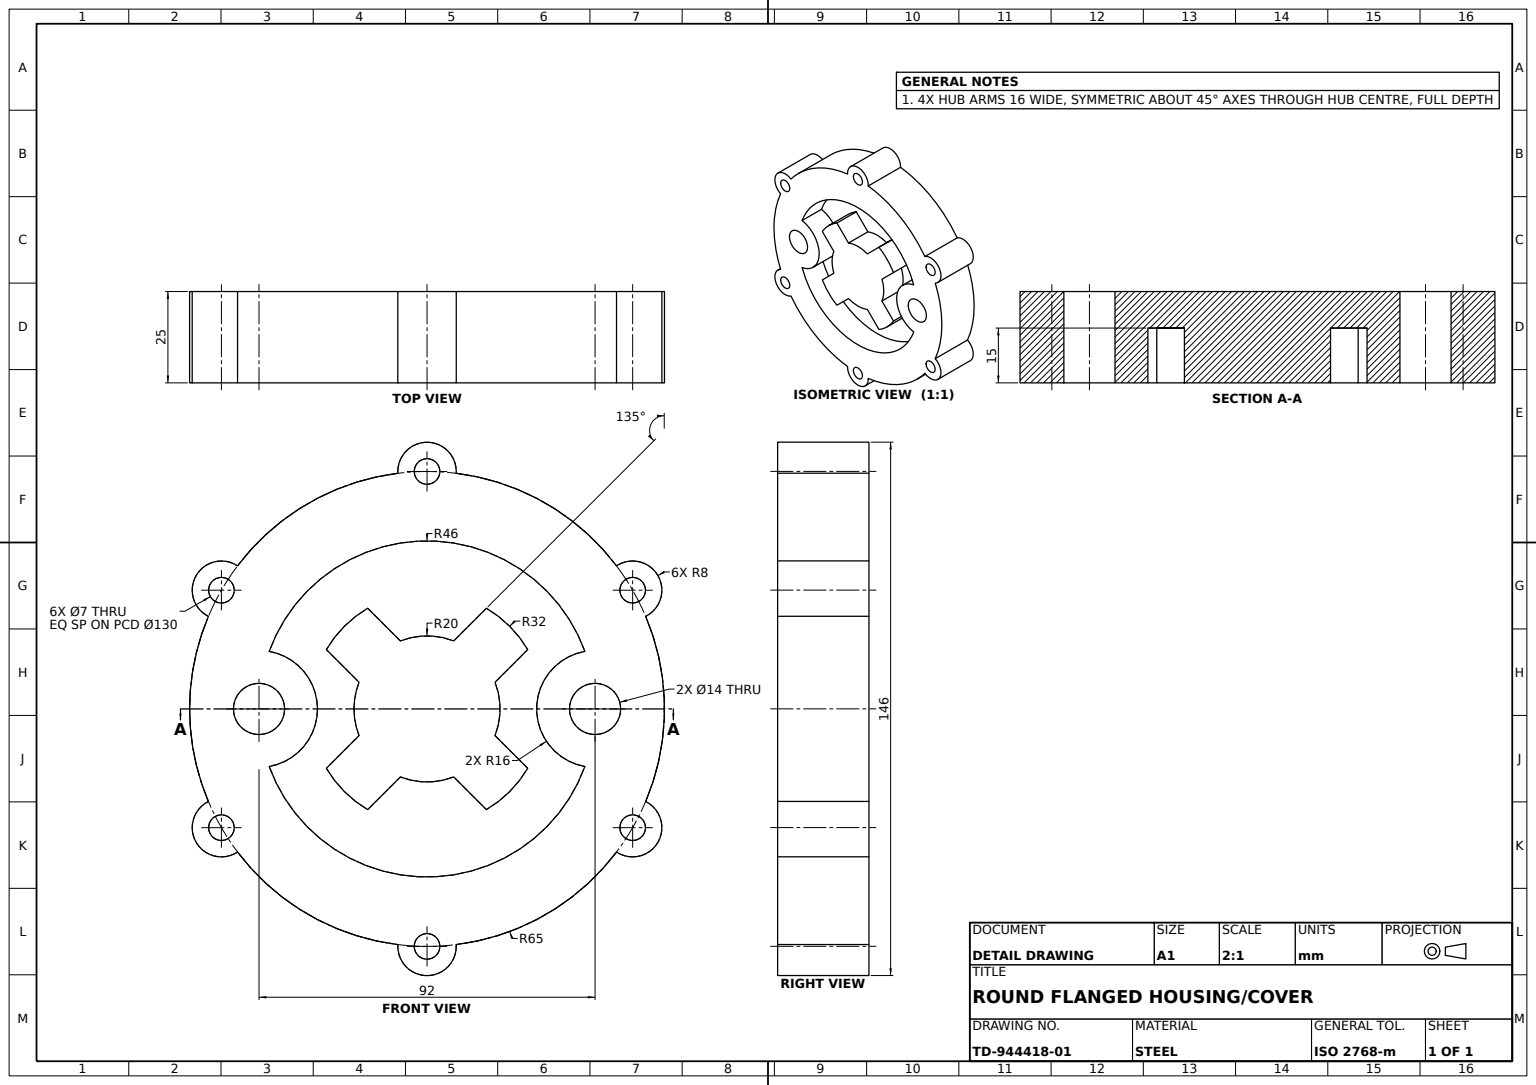
SolidWorks part; units mm, degrees
material "Plain Carbon Steel"
ref_plane "Front Plane" through (0, 0, 0) normal (0, 0, 1) x (1, 0, 0)
ref_plane "Top Plane" through (0, 0, 0) normal (0, 1, 0) x (1, 0, 0)
ref_plane "Right Plane" through (0, 0, 0) normal (1, 0, 0) x (0, 0, -1)
sketch "Flange Profile Sketch" plane through (0, 0, 0) normal (0, 0, 1) x (1, 0, 0)
  arc A0 (-7.9848, 64.5077) -> (-51.8729, 39.1689) centre (0, 0) ccw
  arc A1 (7.9848, 64.5077) -> (-7.9848, 64.5077) centre (0, 65) ccw
  arc A2 (59.8577, 25.3388) -> (51.8729, 39.1689) centre (56.2917, 32.5) ccw
  arc A3 (51.8729, -39.1689) -> (59.8577, -25.3388) centre (56.2917, -32.5) ccw
  arc A4 (-7.9848, -64.5077) -> (7.9848, -64.5077) centre (0, -65) ccw
  arc A5 (-59.8577, -25.3388) -> (-51.8729, -39.1689) centre (-56.2917, -32.5) ccw
  arc A6 (-51.8729, 39.1689) -> (-59.8577, 25.3388) centre (-56.2917, 32.5) ccw
  circle A7 centre (0, 65) radius 3.5
  circle A8 centre (56.2917, 32.5) radius 3.5
  circle A9 centre (56.2917, -32.5) radius 3.5
  circle A10 centre (0, -65) radius 3.5
  circle A11 centre (-56.2917, -32.5) radius 3.5
  circle A12 centre (-56.2917, 32.5) radius 3.5
  arc A13 (51.8729, 39.1689) -> (7.9848, 64.5077) centre (0, 0) ccw
  arc A14 (59.8577, -25.3388) -> (59.8577, 25.3388) centre (0, 0) ccw
  arc A15 (-51.8729, -39.1689) -> (-7.9848, -64.5077) centre (0, 0) ccw
  arc A16 (7.9848, -64.5077) -> (51.8729, -39.1689) centre (0, 0) ccw
  arc A17 (-59.8577, 25.3388) -> (-59.8577, -25.3388) centre (0, 0) ccw
  point P17 (0, 0)
  point P29 (0, 0)
  dimension "D1" = 6
  dimension "D2" = 6
  dimension "D3" = 65
  dimension "D4" = 8
  dimension "D5" = 7
extrude "Flange Body 25mm" add sketch "Flange Profile Sketch" along normal blind 25
sketch "Through Holes Sketch" plane through (0, 0, 25) normal (0, 0, 1) x (1, 0, 0)
  line L0 (0, 0) -> (65, 0) construction
  line L1 (0, 0) -> (0, -68.5) construction
  arc A0 (59.8577, -25.3388) -> (59.8577, 25.3388) centre (0, 0) ccw construction
  circle A1 centre (0, -65) radius 3.5 construction
  circle A2 centre (0, 0) radius 46 construction
  circle A3 centre (46, 0) radius 7
  circle A4 centre (-46, 0) radius 7
  dimension "D1" = 14
  dimension "D2" = 92
extrude "Through Holes" cut sketch "Through Holes Sketch" against normal blind 25
sketch "Annular Pocket Sketch" plane through (0, 0, 25) normal (0, 0, 1) x (1, 0, 0)
  line L0 (0, 0) -> (0, -65) construction
  arc A0 (43.2174, 15.7562) -> (-43.2174, 15.7562) centre (0, 0) ccw
  arc A1 (43.2174, 15.7562) -> (43.2174, -15.7562) centre (46, 0) ccw
  arc A2 (-43.2174, 15.7562) -> (-43.2174, -15.7562) centre (-46, 0) cw
  arc A3 (-43.2174, -15.7562) -> (43.2174, -15.7562) centre (0, 0) ccw
  dimension "D1" = 46
  dimension "D2" = 16
extrude "Annular Pocket 15mm" cut sketch "Annular Pocket Sketch" against normal blind 15
sketch "Cross Hub Sketch" plane through (0, 0, 10) normal (0, 0, 1) x (1, 0, 0)
  line L0 (0, 0) -> (0, -73) construction
  line L1 (-7.3046, 18.6183) -> (-16.252, 27.5658)
  line L2 (-18.6183, -7.3046) -> (-27.5658, -16.252)
  line L3 (-18.6183, 7.3046) -> (-27.5658, 16.252)
  line L4 (-7.3046, -18.6183) -> (-16.252, -27.5658)
  line L5 (18.6183, 7.3046) -> (27.5658, 16.252)
  line L6 (7.3046, 18.6183) -> (16.252, 27.5658)
  line L7 (7.3046, -18.6183) -> (16.252, -27.5658)
  line L8 (18.6183, -7.3046) -> (27.5658, -16.252)
  arc A0 (-7.3046, -18.6183) -> (7.3046, -18.6183) centre (0, 0) ccw
  arc A1 (-7.9848, -64.5077) -> (7.9848, -64.5077) centre (0, -65) ccw construction
  arc A2 (-27.5658, -16.252) -> (-16.252, -27.5658) centre (0, 0) ccw
  arc A3 (-16.252, 27.5658) -> (-27.5658, 16.252) centre (0, 0) ccw
  arc A4 (27.5658, 16.252) -> (16.252, 27.5658) centre (0, 0) ccw
  arc A5 (16.252, -27.5658) -> (27.5658, -16.252) centre (0, 0) ccw
  arc A6 (-18.6183, 7.3046) -> (-18.6183, -7.3046) centre (0, 0) ccw
  arc A7 (7.3046, 18.6183) -> (-7.3046, 18.6183) centre (0, 0) ccw
  arc A8 (18.6183, -7.3046) -> (18.6183, 7.3046) centre (0, 0) ccw
  point P3 (-5.6569, 5.6569)
  point P8 (-55.0353, -55.0353)
  point P9 (-60.6922, -49.3784)
  point P10 (5.6569, -5.6569)
  point P11 (-49.3784, -60.6922)
  point P30 (0, 0)
  dimension "D1" = 4
  dimension "D4" = 15.6516
  dimension "D2" = 20
  dimension "D3" = 32
extrude "Cross Hub 15mm" add sketch "Cross Hub Sketch" along normal blind 15
